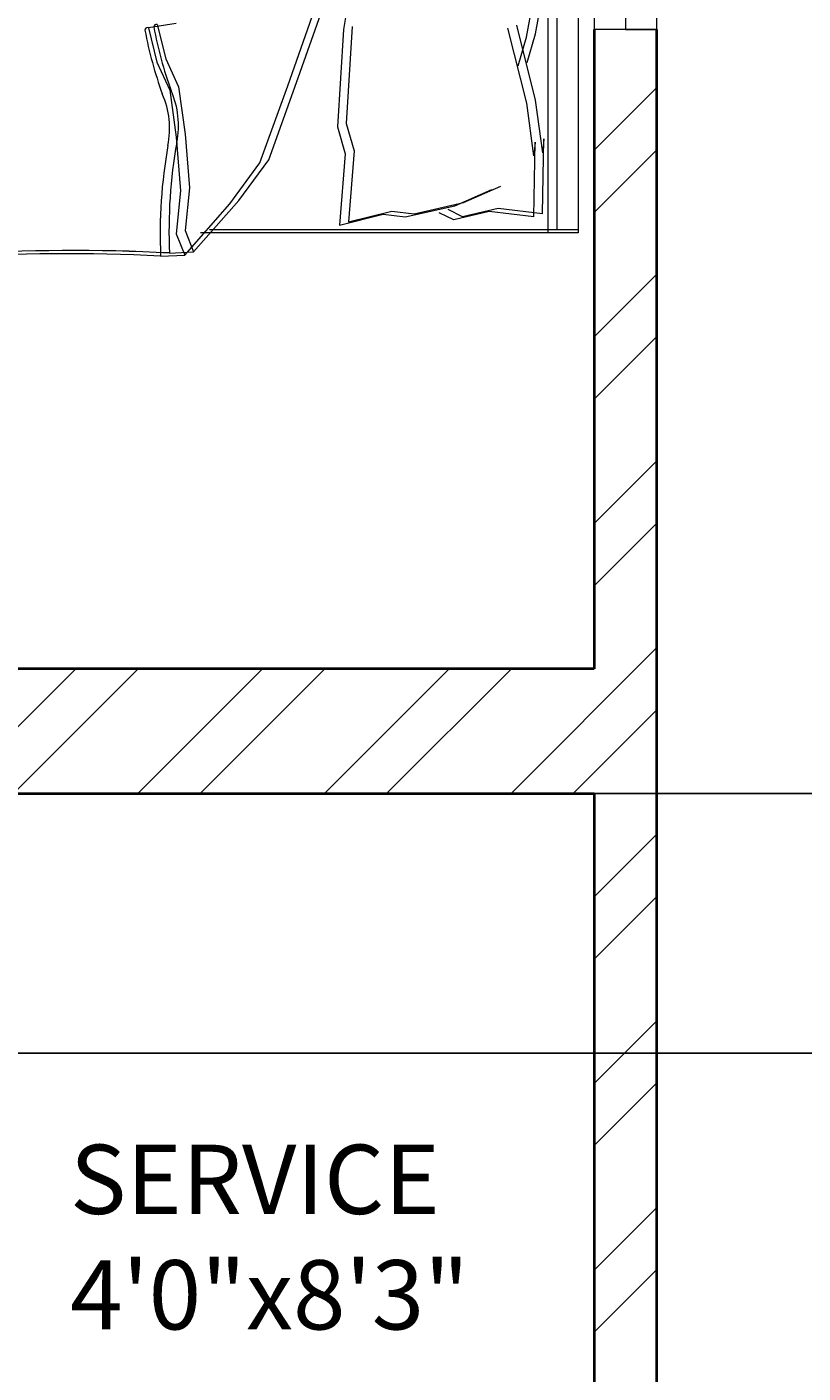
# Model space of a CAD drawing. Units: inches. Extents: x 1601 to 2297, y 1496 to 2631.
# Tile 31 of 57: x 2185 to 2241, y 2043 to 2141. Entities that reach past the tile are written whole.
import ezdxf

# ---------------------------------------------------------------- set-up
doc = ezdxf.new("R2010")
doc.units = ezdxf.units.IN
for name, color, linetype, lineweight in [('A-ANNO-DIMS', 2, 'Continuous', 18), ('A-AREA-IDEN', 7, 'Continuous', 18), ('A-FURN', 8, 'Continuous', 18), ('A-GLAZ', 161, 'Continuous', 20), ('A-WALL', 7, 'Continuous', 40), ('A-WALL-PATT', 215, 'Continuous', 13)]:
    doc.layers.add(name, color=color, linetype=linetype, lineweight=lineweight)
doc.styles.get("Standard").update_dxf_attribs({"font": 'arial.ttf'})
doc.dimstyles.get("Standard").update_dxf_attribs({"dimtxt": 0.18, "dimasz": 0.18, "dimexe": 0.18, "dimexo": 0.0625, "dimgap": 0.09, "dimtad": 0, "dimtih": 1, "dimtoh": 1, "dimdec": 4, "dimzin": 0, "dimdsep": 46, "dimtxsty": 'Standard', "dimcen": 0.09, "dimadec": 0, "dimazin": 0, "dimtfac": 1, "dimtdec": 4, "dimtofl": 0, "dimtmove": 0, "dimatfit": 3, "dimfxl": 1, "dimtolj": 1, "dimtzin": 0, "dimarcsym": 0})

# ---------------------------------------------------------------- blocks, each defined once
blk = doc.blocks.new('BED-DOUBLE')
for p, q in [((27.746, 52.867), (24.495, 49.162)), ((27.746, 52.867), (24.495, 49.162)), ((27.746, 52.867), (24.495, 49.162)), ((27.746, 52.867), (24.495, 49.162)), ((28.385, 53.096), (25.135, 49.39)), ((28.385, 53.096), (25.135, 49.39)), ((28.385, 53.096), (25.135, 49.39)), ((28.385, 53.096), (25.135, 49.39)), ((29.49, 52.947), (27.746, 52.867, 3.871)), ((29.49, 52.947), (27.746, 52.867, 3.871)), ((29.49, 52.947), (27.746, 52.867, 3.871)), ((29.49, 52.947), (27.746, 52.867, 3.871)), ((28.365, 51.33), (27.746, 52.867)), ((28.365, 51.33), (27.746, 52.867)), ((28.365, 51.33), (27.746, 52.867)), ((28.365, 51.33), (27.746, 52.867)), ((30.13, 53.175), (28.385, 53.096, 3.871)), ((30.13, 53.175), (28.385, 53.096, 3.871)), ((30.13, 53.175), (28.385, 53.096, 3.871)), ((30.13, 53.175), (28.385, 53.096, 3.871)), ((29.004, 51.559), (28.385, 53.096)), ((29.004, 51.558), (28.385, 53.096)), ((29.004, 51.559), (28.385, 53.096)), ((29.004, 51.558), (28.385, 53.096)), ((28.695, 48.461), (29.004, 51.559)), ((28.695, 48.461), (29.004, 51.559)), ((28.695, 48.461), (29.004, 51.558)), ((28.695, 48.461), (29.004, 51.558)), ((0, 51.494), (0.639, 51.493)), ((0, 3.475), (0, 51.494)), ((0, 51.494), (0.639, 51.493)), ((0, 3.475), (0, 51.494)), ((0, 51.265), (26.61, 51.265)), ((0, 51.265), (26.61, 51.265)), ((0, 51.265), (26.61, 51.265)), ((0, 51.265), (26.61, 51.265)), ((0.639, 51.494), (27.249, 51.494)), ((0.639, 51.494), (27.249, 51.494)), ((0.639, 51.493), (27.249, 51.493)), ((0.639, 51.493), (27.249, 51.493)), ((1.533, 3.475), (1.533, 51.265)), ((1.533, 3.475), (1.533, 51.265)), ((1.533, 3.475), (1.533, 51.265)), ((1.533, 3.475), (1.533, 51.265)), ((2.173, 3.703), (2.173, 51.494)), ((2.173, 3.703), (2.173, 51.494)), ((2.173, 3.703), (2.173, 51.493)), ((2.173, 3.703), (2.173, 51.493)), ((6.407, 49.961), (8.977, 50.557)), ((6.407, 49.961), (8.977, 50.557)), ((6.407, 49.961), (8.977, 50.556)), ((6.407, 49.961), (8.977, 50.556)), ((8.977, 50.557), (10.024, 50.043)), ((8.977, 50.557), (10.024, 50.043)), ((8.977, 50.556), (10.024, 50.042)), ((8.977, 50.556), (10.024, 50.042)), ((16.573, 50.698), (13.434, 49.923)), ((16.573, 50.698), (13.434, 49.922)), ((16.573, 50.698), (13.434, 49.923)), ((16.573, 50.698), (13.434, 49.922)), ((17.212, 50.926), (14.073, 50.151)), ((17.212, 50.926), (14.073, 50.151)), ((17.212, 50.926), (14.073, 50.151)), ((17.212, 50.926), (14.073, 50.151)), ((16.169, 45.566), (16.573, 50.698)), ((16.169, 45.566), (16.573, 50.698)), ((16.169, 45.566), (16.573, 50.698)), ((16.169, 45.566), (16.573, 50.698)), ((16.808, 45.795), (17.212, 50.926)), ((16.808, 45.794), (17.212, 50.926)), ((16.808, 45.795), (17.212, 50.926)), ((16.808, 45.794), (17.212, 50.926)), ((28.055, 48.233), (28.365, 51.33)), ((28.055, 48.233), (28.365, 51.33)), ((28.055, 48.233), (28.365, 51.33)), ((28.055, 48.233), (28.365, 51.33)), ((2.557, 50.112), (2.46, 44.709)), ((2.557, 50.112), (2.46, 44.709)), ((2.557, 50.111), (2.46, 44.709)), ((2.557, 50.111), (2.46, 44.709)), ((2.557, 50.112), (5.768, 49.733)), ((2.557, 50.112), (5.768, 49.733)), ((2.557, 50.111), (5.768, 49.733)), ((2.557, 50.111), (5.768, 49.733)), ((3.196, 50.34), (3.099, 44.938)), ((3.196, 50.34), (3.099, 44.938)), ((3.196, 50.34), (3.099, 44.938)), ((3.196, 50.34), (3.099, 44.938)), ((3.196, 50.34), (6.407, 49.961)), ((3.196, 50.34), (6.407, 49.961)), ((3.196, 50.34), (6.407, 49.961)), ((3.196, 50.34), (6.407, 49.961)), ((5.768, 49.733), (8.338, 50.328)), ((5.768, 49.733), (8.338, 50.328)), ((5.768, 49.733), (8.338, 50.328)), ((5.768, 49.733), (8.338, 50.328)), ((11.829, 50.112), (8.257, 49.309)), ((11.829, 50.112), (8.257, 49.309)), ((11.829, 50.112), (8.257, 49.309)), ((11.829, 50.112), (8.257, 49.309)), ((8.338, 50.328), (9.384, 49.814)), ((8.338, 50.328), (9.384, 49.814)), ((8.338, 50.328), (9.384, 49.814)), ((8.338, 50.328), (9.384, 49.814)), ((12.468, 50.34), (8.896, 49.538)), ((12.468, 50.34), (8.896, 49.537)), ((12.468, 50.34), (8.896, 49.538)), ((12.468, 50.34), (8.896, 49.537)), ((13.434, 49.923), (11.829, 50.112)), ((13.434, 49.922), (11.829, 50.112)), ((13.434, 49.923), (11.829, 50.112)), ((13.434, 49.922), (11.829, 50.112)), ((14.073, 50.151), (12.468, 50.34)), ((14.073, 50.151), (12.468, 50.34)), ((14.073, 50.151), (12.468, 50.34)), ((14.073, 50.151), (12.468, 50.34)), ((8.257, 49.309), (5.578, 48.128)), ((8.257, 49.309), (5.578, 48.128)), ((8.257, 49.309), (5.578, 48.128)), ((8.257, 49.309), (5.578, 48.128)), ((8.896, 49.538), (6.218, 48.356)), ((8.896, 49.538), (6.218, 48.356)), ((8.896, 49.537), (6.218, 48.356)), ((8.896, 49.537), (6.218, 48.356)), ((24.495, 49.162), (22.329, 46.219)), ((24.495, 49.162), (22.329, 46.219)), ((24.495, 49.162), (22.329, 46.219)), ((24.495, 49.162), (22.329, 46.219)), ((25.135, 49.39), (22.968, 46.448)), ((25.135, 49.39), (22.968, 46.448)), ((25.135, 49.39), (22.968, 46.448)), ((25.135, 49.39), (22.968, 46.448)), ((28.365, 44.361), (28.055, 48.233)), ((28.365, 44.361), (28.055, 48.233)), ((28.365, 44.361), (28.055, 48.233)), ((28.365, 44.361), (28.055, 48.233)), ((29.004, 44.589), (28.695, 48.461)), ((29.004, 44.589), (28.695, 48.461)), ((29.004, 44.589), (28.695, 48.461)), ((29.004, 44.589), (28.695, 48.461)), ((2.46, 44.709), (2.542, 45.712)), ((2.46, 44.709), (2.542, 45.712)), ((2.46, 44.709), (2.542, 45.712)), ((2.46, 44.709), (2.542, 45.712)), ((2.542, 45.712), (3.069, 41.914)), ((2.542, 45.712), (3.069, 41.914)), ((2.542, 45.712), (3.069, 41.914)), ((2.542, 45.712), (3.069, 41.914)), ((3.099, 44.938), (3.181, 45.941)), ((3.099, 44.938), (3.181, 45.941)), ((3.099, 44.938), (3.181, 45.94)), ((3.099, 44.938), (3.181, 45.94)), ((3.181, 45.941), (3.709, 42.143)), ((3.181, 45.941), (3.709, 42.143)), ((3.181, 45.94), (3.709, 42.142)), ((3.181, 45.94), (3.709, 42.142)), ((17.365, 43.834), (16.808, 45.795)), ((17.365, 43.834), (16.808, 45.795)), ((17.365, 43.834), (16.808, 45.794)), ((17.365, 43.834), (16.808, 45.794)), ((22.329, 46.219), (20.316, 40.644)), ((22.329, 46.219), (20.316, 40.644)), ((22.329, 46.219), (20.317, 40.644)), ((22.329, 46.219), (20.317, 40.644)), ((22.968, 46.448), (20.956, 40.872)), ((22.968, 46.448), (20.956, 40.872)), ((22.968, 46.448), (20.956, 40.872)), ((22.968, 46.448), (20.956, 40.872)), ((16.726, 43.606), (16.169, 45.566)), ((16.726, 43.606), (16.169, 45.566)), ((16.726, 43.606), (16.169, 45.566)), ((16.726, 43.606), (16.169, 45.566)), ((16.934, 36.824), (17.365, 43.834)), ((16.934, 36.824), (17.365, 43.834)), ((16.934, 36.824), (17.365, 43.834)), ((16.934, 36.824), (17.365, 43.834)), ((28.829, 40.954), (28.365, 44.361)), ((28.829, 40.953), (28.365, 44.361)), ((28.829, 40.954), (28.365, 44.361)), ((28.829, 40.953), (28.365, 44.361)), ((29.468, 41.182), (29.004, 44.589)), ((29.469, 41.182), (29.004, 44.589)), ((29.468, 41.182), (29.004, 44.589)), ((29.469, 41.182), (29.004, 44.589)), ((16.295, 36.596), (16.726, 43.606)), ((16.295, 36.596), (16.726, 43.606)), ((16.295, 36.596), (16.726, 43.606)), ((16.295, 36.596), (16.726, 43.606)), ((3.069, 41.914), (4.422, 36.495)), ((3.069, 41.914), (4.422, 36.495)), ((3.069, 41.914), (4.422, 36.495)), ((3.069, 41.914), (4.422, 36.495)), ((3.709, 42.143), (5.061, 36.723)), ((3.709, 42.143), (5.061, 36.723)), ((3.709, 42.142), (5.061, 36.723)), ((3.709, 42.142), (5.061, 36.723)), ((20.956, 40.872), (18.022, 32.534)), ((20.956, 40.872), (18.022, 32.534)), ((20.956, 40.872), (18.022, 32.534)), ((20.956, 40.872), (18.022, 32.534)), ((29.758, 38.94), (28.829, 40.954)), ((29.758, 38.94), (28.829, 40.954)), ((29.758, 38.94), (28.829, 40.953)), ((29.758, 38.94), (28.829, 40.953)), ((30.397, 39.169), (29.468, 41.182)), ((30.397, 39.169), (29.468, 41.182)), ((30.397, 39.168), (29.469, 41.182)), ((30.397, 39.168), (29.469, 41.182)), ((20.316, 40.644), (17.383, 32.306)), ((20.317, 40.644), (17.383, 32.306)), ((20.316, 40.644), (17.383, 32.306)), ((20.317, 40.644), (17.383, 32.306)), ((3.673, 39.2), (3.078, 37.135)), ((3.673, 39.2), (3.078, 37.135)), ((3.673, 39.2), (3.078, 37.135)), ((3.673, 39.2), (3.078, 37.135)), ((4.313, 39.428), (3.717, 37.363)), ((4.313, 39.428), (3.717, 37.363)), ((4.313, 39.428), (3.718, 37.363)), ((4.313, 39.428), (3.718, 37.363)), ((30.377, 36.462), (29.758, 38.94)), ((30.377, 36.462), (29.758, 38.94)), ((30.377, 36.462), (29.758, 38.94)), ((30.377, 36.462), (29.758, 38.94)), ((31.016, 36.691), (30.397, 39.169)), ((31.016, 36.691), (30.397, 39.169)), ((31.016, 36.691), (30.397, 39.168)), ((31.016, 36.691), (30.397, 39.168)), ((3.078, 37.135), (2.537, 34.204)), ((3.078, 37.135), (2.537, 34.204)), ((3.078, 37.135), (2.537, 34.204)), ((3.078, 37.135), (2.537, 34.204)), ((3.717, 37.363), (3.176, 34.433)), ((3.718, 37.363), (3.176, 34.433)), ((3.717, 37.363), (3.176, 34.433)), ((3.718, 37.363), (3.176, 34.433)), ((16.268, 32.792), (16.934, 36.824)), ((16.268, 32.792), (16.934, 36.824)), ((16.268, 32.792), (16.934, 36.824)), ((16.268, 32.792), (16.934, 36.824)), ((29.004, 36.381), (31.016, 36.691)), ((29.004, 36.381), (31.016, 36.691)), ((29.004, 36.381), (31.016, 36.691)), ((29.004, 36.381), (31.016, 36.691))]:
    blk.add_line(p, q)
for centre, radius, start, end in [((-6.656, 51.327), 36.183, 349.87628, 2.56571), ((-6.656, 51.327), 36.183, 349.87628, 2.56571), ((-6.656, 51.327), 36.183, 349.87628, 2.56571), ((-6.656, 51.327), 36.183, 349.87628, 2.56571), ((36.315, 182.266), 129.499, 266.97912, 273.83645), ((36.315, 182.265), 129.499, 266.97912, 273.83645), ((36.315, 182.266), 129.499, 266.97912, 273.83645), ((36.315, 182.265), 129.499, 266.97912, 273.83645), ((-6.017, 51.555), 36.183, 349.87628, 2.56571), ((-6.017, 51.555), 36.183, 349.87628, 2.56571), ((-6.017, 51.555), 36.183, 349.87628, 2.56571), ((-6.017, 51.555), 36.183, 349.87628, 2.56571), ((36.954, 182.494), 129.499, 266.97912, 273.83645), ((36.954, 182.494), 129.499, 266.97912, 273.83645), ((36.954, 182.494), 129.499, 266.97912, 273.83645), ((36.954, 182.494), 129.499, 266.97912, 273.83645), ((35.066, 43.743), 6.224, 168.6608, 203.73842), ((35.066, 43.743), 6.224, 168.6608, 203.73842), ((35.066, 43.743), 6.224, 168.6608, 203.73842), ((35.066, 43.743), 6.224, 168.6608, 203.73842), ((35.705, 43.972), 6.224, 168.6608, 203.73842), ((35.705, 43.971), 6.224, 168.6608, 203.73842), ((35.705, 43.972), 6.224, 168.6608, 203.73842), ((35.705, 43.971), 6.224, 168.6608, 203.73842), ((1.482, 31.154), 29.654, 10.66171, 19.88058), ((1.482, 31.154), 29.654, 10.66171, 19.88058), ((1.482, 31.153), 29.654, 10.66171, 19.88058), ((1.482, 31.153), 29.654, 10.66171, 19.88058), ((2.121, 31.382), 29.654, 10.66171, 19.88058), ((2.121, 31.382), 29.654, 10.66171, 19.88058), ((2.121, 31.382), 29.654, 10.66171, 19.88058), ((2.121, 31.382), 29.654, 10.66171, 19.88058), ((30.439, 36.636), 0.185, 250.24637, 1.13765), ((30.439, 36.636), 0.185, 250.24637, 1.13765), ((30.439, 36.636), 0.185, 250.24637, 1.13765), ((30.439, 36.636), 0.185, 250.24637, 1.13765), ((31.079, 36.864), 0.185, 250.24637, 1.13765), ((31.079, 36.864), 0.185, 250.24637, 1.13765), ((31.079, 36.864), 0.185, 250.24637, 1.13765), ((31.079, 36.864), 0.185, 250.24637, 1.13765)]:
    blk.add_arc(centre, radius, start, end)
blk = doc.blocks.new('WIN-60IN-JAMB4P5')
for p, q in [((0, 60), (4.5, 60)), ((0, 60), (0, 0)), ((4.5, 60), (2.25, 60)), ((2.25, 60), (2.25, 0)), ((4.5, 60), (4.5, 0)), ((4.5, 0), (0, 0)), ((2.25, 0), (4.5, 0))]:
    blk.add_line(p, q)
blk = doc.blocks.new('*D29')
at = {"layer": 'A-ANNO-DIMS', "color": 0, "lineweight": -2, "transparency": 16777216}
for p, q in [((2230.6, 2532.325), (2279.267, 2532.325)), ((2279.087, 2532.145), (2279.087, 2084.007)), ((2279.087, 1635.505), (2279.087, 2083.643)), ((2230.6, 1635.325), (2279.267, 1635.325))]:
    blk.add_line(p, q, dxfattribs=at)
at = {"layer": 'A-ANNO-DIMS', "color": 0, "transparency": 16777216}
for points in [[(2279.057, 2532.145), (2279.117, 2532.145), (2279.087, 2532.325)], [(2279.057, 1635.505), (2279.117, 1635.505), (2279.087, 1635.325)]]:
    blk.add_solid(points, dxfattribs=at)
at = {"layer": 'Defpoints', "color": 0, "transparency": 16777216}
for p in [(2230.537, 2532.325), (2279.087, 2532.325), (2230.537, 1635.325)]:
    blk.add_point(p, dxfattribs=at)
at = {"layer": 'A-ANNO-DIMS', "color": 0, "transparency": 16777216, "insert": (2279.087, 2083.825), "char_height": 0.18, "attachment_point": 5}
blk.add_mtext('\\A1;897', dxfattribs=at)
blk = doc.blocks.new('*D37')
at = {"layer": 'A-ANNO-DIMS', "color": 0, "lineweight": -2, "transparency": 16777216}
for p, q in [((2040.1, 2085.325), (2279.267, 2085.325)), ((2279.087, 2085.145), (2279.087, 2076.132)), ((2279.087, 2066.755), (2279.087, 2075.768)), ((2040.1, 2066.575), (2279.267, 2066.575))]:
    blk.add_line(p, q, dxfattribs=at)
at = {"layer": 'A-ANNO-DIMS', "color": 0, "transparency": 16777216}
for points in [[(2279.057, 2085.145), (2279.117, 2085.145), (2279.087, 2085.325)], [(2279.057, 2066.755), (2279.117, 2066.755), (2279.087, 2066.575)]]:
    blk.add_solid(points, dxfattribs=at)
at = {"layer": 'Defpoints', "color": 0, "transparency": 16777216}
for p in [(2040.037, 2085.325), (2279.087, 2085.325), (2040.037, 2066.575)]:
    blk.add_point(p, dxfattribs=at)
at = {"layer": 'A-ANNO-DIMS', "color": 0, "transparency": 16777216, "insert": (2279.087, 2075.95), "char_height": 0.18, "attachment_point": 5}
blk.add_mtext('\\A1;18.75', dxfattribs=at)

msp = doc.modelspace()

# ---------------------------------------------------------------- hatches: boundary and pattern name
at = {"layer": 'A-WALL-PATT'}
h = msp.add_hatch(dxfattribs=at)
h.set_pattern_fill('ANSI32', color=256)
h.paths.add_polyline_path([(1842.0336, 2528.0767), (1842.0336, 2532.3254), (1686.0373, 2532.3254), (1686.0373, 2492.9493), (1695.0373, 2492.9493), (1695.0373, 2523.3254), (1827.0373, 2523.3254), (1827.0373, 2416.8254), (1834.6225, 2416.8254), (1834.6225, 2419.0754), (1834.6225, 2421.3254), (1831.5373, 2421.3254), (1831.5373, 2523.3254), (1842.0336, 2523.3254)])
h.paths.add_polyline_path([(1695.0373, 2432.9493), (1686.0373, 2432.9493), (1686.0373, 2325.989), (1695.0373, 2325.989), (1695.0373, 2347.8254), (1827.0373, 2347.8254), (1827.0373, 2287.8254), (1823.2991, 2287.8254), (1823.2991, 2283.3254), (1847.9422, 2283.3254), (1847.9422, 2285.5754), (1847.9422, 2287.8254), (1831.5373, 2287.8254), (1831.5373, 2347.8254), (1846.9946, 2347.8254), (1846.9946, 2350.0754), (1846.9946, 2352.3254), (1695.0373, 2352.3254)])
h.paths.add_polyline_path([(1807.1169, 1573.5395), (2055.0405, 1573.5395), (2055.0405, 1610.6322), (1807.1169, 1610.6322)], flags=9)
h.paths.add_polyline_path([(1841.1631, 1712.7967), (1870.3957, 1712.7967), (1870.3957, 1731.454), (1841.1631, 1731.454)], flags=9)
h.paths.add_polyline_path([(2144.3862, 1772.185), (2191.0233, 1772.185), (2191.0233, 1790.8423), (2144.3862, 1790.8423)], flags=9)
h.paths.add_polyline_path([(2143.0128, 1827.3312), (2177.9958, 1827.3312), (2177.9958, 1845.9886), (2143.0128, 1845.9886)], flags=9)
h.paths.add_polyline_path([(2041.2439, 1833.5691), (2070.8516, 1833.5691), (2070.8516, 1852.2264), (2041.2439, 1852.2264)], flags=9)
h.paths.add_polyline_path([(2097.2791, 1947.0598), (2134.2061, 1947.0598), (2134.2061, 1965.7171), (2097.2791, 1965.7171)], flags=9)
h.paths.add_polyline_path([(2214.995, 1904.3124), (2214.995, 1942.2899), (2196.3376, 1942.2899), (2196.3376, 1904.3124)], flags=9)
h.paths.add_polyline_path([(2186.6284, 2043.8031), (2219.7935, 2043.8031), (2219.7935, 2062.4605), (2186.6284, 2062.4605)], flags=9)
h.paths.add_polyline_path([(2064.0877, 2031.616), (2097.4949, 2031.616), (2097.4949, 2050.2734), (2064.0877, 2050.2734)], flags=9)
h.paths.add_polyline_path([(1973.1349, 1986.0688), (2008.4009, 1986.0688), (2008.4009, 2004.7261), (1973.1349, 2004.7261)], flags=9)
h.paths.add_polyline_path([(1976.3676, 2106.9635), (2005.7469, 2106.9635), (2005.7469, 2125.6209), (1976.3676, 2125.6209)], flags=9)
h.paths.add_polyline_path([(1991.7852, 2180.4863), (2027.0513, 2180.4863), (2027.0513, 2199.1437), (1991.7852, 2199.1437)], flags=9)
h.paths.add_polyline_path([(2106.1801, 2187.9359), (2152.2101, 2187.9359), (2152.2101, 2206.5932), (2106.1801, 2206.5932)], flags=9)
h.paths.add_polyline_path([(2148.6686, 2262.2542), (2182.318, 2262.2542), (2182.318, 2280.9115), (2148.6686, 2280.9115)], flags=9)
h.paths.add_polyline_path([(2041.6327, 2252.8147), (2071.2405, 2252.8147), (2071.2405, 2271.4721), (2041.6327, 2271.4721)], flags=9)
h.paths.add_polyline_path([(2063.9734, 2375.4265), (2100.9004, 2375.4265), (2100.9004, 2394.0839), (2063.9734, 2394.0839)], flags=9)
h.paths.add_polyline_path([(2216.4955, 2330.9748), (2216.4955, 2370.2654), (2197.8381, 2370.2654), (2197.8381, 2330.9748)], flags=9)
h.paths.add_polyline_path([(2179.1416, 2485.8687), (2212.3067, 2485.8687), (2212.3067, 2504.5261), (2179.1416, 2504.5261)], flags=9)
h.paths.add_polyline_path([(2078.7442, 2471.1516), (2112.1514, 2471.1516), (2112.1514, 2489.809), (2078.7442, 2489.809)], flags=9)
h.paths.add_polyline_path([(1915.9631, 2329.4668), (1952.8902, 2329.4668), (1952.8902, 2348.1241), (1915.9631, 2348.1241)], flags=9)
h.paths.add_polyline_path([(1904.3189, 2499.6709), (1940.4512, 2499.6709), (1940.4512, 2518.3282), (1904.3189, 2518.3282)], flags=9)
h.paths.add_polyline_path([(1892.3665, 2100.4595), (1925.6374, 2100.4595), (1925.6374, 2119.1169), (1892.3665, 2119.1169)], flags=9)
h.paths.add_polyline_path([(1909.2984, 1805.9631), (1946.2254, 1805.9631), (1946.2254, 1824.6205), (1909.2984, 1824.6205)], flags=9)
h.paths.add_polyline_path([(1934.6056, 1658.616), (1970.738, 1658.616), (1970.738, 1677.2733), (1934.6056, 1677.2733)], flags=9)
h.paths.add_polyline_path([(1711.2052, 1789.8902), (1750.0456, 1789.8902), (1750.0456, 1808.5476), (1711.2052, 1808.5476)], flags=9)
h.paths.add_polyline_path([(1742.7874, 1854.6743), (1771.9449, 1854.6743), (1771.9449, 1873.3317), (1742.7874, 1873.3317)], flags=9)
h.paths.add_polyline_path([(1807.3592, 1997.7912), (1850.1116, 1997.7912), (1850.1116, 2016.4486), (1807.3592, 2016.4486)], flags=9)
h.paths.add_polyline_path([(1717.4579, 2237.7844), (1760.2103, 2237.7844), (1760.2103, 2256.4417), (1717.4579, 2256.4417)], flags=9)
h.paths.add_polyline_path([(1780.9285, 2324.0623), (1810.086, 2324.0623), (1810.086, 2342.7197), (1780.9285, 2342.7197)], flags=25)
h.paths.add_polyline_path([(1837.696, 2449.2024), (1866.9286, 2449.2024), (1866.9286, 2467.8598), (1837.696, 2467.8598)], flags=9)
h.paths.add_polyline_path([(1712.7752, 2484.9404), (1751.6156, 2484.9404), (1751.6156, 2503.5977), (1712.7752, 2503.5977)], flags=25)
h = msp.add_hatch(dxfattribs=at)
h.set_pattern_fill('ANSI32', color=256)
h.paths.add_polyline_path([(1973.9371, 2211.3254), (1893.0373, 2211.3254), (1893.0373, 2287.8254), (1884.6167, 2287.8254), (1884.6167, 2285.5754), (1884.6167, 2283.3254), (1888.5373, 2283.3254), (1888.5373, 2145.3254), (1695.0373, 2145.3254), (1695.0373, 2173.8724), (1690.5373, 2173.8724), (1686.0373, 2173.8724), (1686.0373, 2136.3254), (1722.5687, 2136.3254), (1722.5687, 2117.4352), (1731.5687, 2117.4352), (1731.5687, 2136.3254), (1893.0373, 2136.3254), (1893.0373, 2202.3254), (1959.0373, 2202.3254), (1959.0373, 2182.1303), (1968.0373, 2182.1303), (1968.0373, 2202.3254), (1973.9371, 2202.3254)])
h.paths.add_polyline_path([(2094.0373, 2274.6364), (2096.4294, 2274.6364), (2096.4294, 2276.8864), (2096.4294, 2279.1364), (2094.0373, 2279.1364), (2094.0373, 2290.8254), (2094.0373, 2295.3254), (2089.5373, 2295.3254), (2089.5373, 2230.8254), (2035.5373, 2230.8254), (2035.5373, 2299.8254), (2031.0373, 2299.8254), (2031.0373, 2211.3254), (2023.0065, 2211.3254), (2023.0065, 2202.3254), (2031.0373, 2202.3254), (2031.0373, 2140.8254), (1968.0373, 2140.8254), (1968.0373, 2145.9106), (1963.5373, 2145.9106), (1959.0373, 2145.9106), (1959.0373, 2116.839), (1963.5373, 2116.839), (1968.0373, 2116.839), (1968.0373, 2131.8254), (2031.0373, 2131.8254), (2031.0373, 2094.3254), (2031.0373, 2085.3254), (2031.0373, 2056.8254), (1968.0373, 2056.8254), (1968.0373, 2070.4947), (1963.5373, 2070.4947), (1959.0373, 2070.4947), (1959.0373, 2040.3029), (1968.0373, 2040.3029), (1968.0373, 2047.8254), (2031.0373, 2047.8254), (2031.0373, 1983.3254), (2031.0373, 1978.8254), (2021.1979, 1978.8254), (2021.1979, 1974.3254), (2031.0373, 1974.3254), (2031.0373, 1954.3528), (2035.5373, 1954.3528), (2035.5373, 1974.3254), (2035.5373, 1981.8254), (2055.5513, 1981.8254), (2055.5513, 1986.3254), (2035.5373, 1986.3254), (2035.5373, 2047.8254), (2040.0373, 2047.8254), (2040.0373, 2085.3254), (2040.0373, 2094.3254), (2040.0373, 2140.8254), (2035.5373, 2140.8254), (2035.5373, 2226.3254), (2089.5373, 2226.3254), (2094.0373, 2226.3254)])
h.paths.add_polyline_path([(2226.0373, 2230.8254), (2134.5373, 2230.8254), (2134.5373, 2233.5437), (2130.0373, 2233.5437), (2130.0373, 2226.3254), (2134.5373, 2226.3254), (2226.0373, 2226.3254)])
h.paths.add_polyline_path([(1807.1169, 1573.5395), (2055.0405, 1573.5395), (2055.0405, 1610.6322), (1807.1169, 1610.6322)], flags=9)
h.paths.add_polyline_path([(1841.1631, 1712.7967), (1870.3957, 1712.7967), (1870.3957, 1731.454), (1841.1631, 1731.454)], flags=9)
h.paths.add_polyline_path([(2144.3862, 1772.185), (2191.0233, 1772.185), (2191.0233, 1790.8423), (2144.3862, 1790.8423)], flags=9)
h.paths.add_polyline_path([(2143.0128, 1827.3312), (2177.9958, 1827.3312), (2177.9958, 1845.9886), (2143.0128, 1845.9886)], flags=9)
h.paths.add_polyline_path([(2041.2439, 1833.5691), (2070.8516, 1833.5691), (2070.8516, 1852.2264), (2041.2439, 1852.2264)], flags=9)
h.paths.add_polyline_path([(2097.2791, 1947.0598), (2134.2061, 1947.0598), (2134.2061, 1965.7171), (2097.2791, 1965.7171)], flags=9)
h.paths.add_polyline_path([(2214.995, 1904.3124), (2214.995, 1942.2899), (2196.3376, 1942.2899), (2196.3376, 1904.3124)], flags=9)
h.paths.add_polyline_path([(2186.6284, 2043.8031), (2219.7935, 2043.8031), (2219.7935, 2062.4605), (2186.6284, 2062.4605)], flags=9)
h.paths.add_polyline_path([(2064.0877, 2031.616), (2097.4949, 2031.616), (2097.4949, 2050.2734), (2064.0877, 2050.2734)], flags=9)
h.paths.add_polyline_path([(1973.1349, 1986.0688), (2008.4009, 1986.0688), (2008.4009, 2004.7261), (1973.1349, 2004.7261)], flags=25)
h.paths.add_polyline_path([(1976.3676, 2106.9635), (2005.7469, 2106.9635), (2005.7469, 2125.6209), (1976.3676, 2125.6209)], flags=25)
h.paths.add_polyline_path([(1991.7852, 2180.4863), (2027.0513, 2180.4863), (2027.0513, 2199.1437), (1991.7852, 2199.1437)], flags=25)
h.paths.add_polyline_path([(2106.1801, 2187.9359), (2152.2101, 2187.9359), (2152.2101, 2206.5932), (2106.1801, 2206.5932)], flags=9)
h.paths.add_polyline_path([(2148.6686, 2262.2542), (2182.318, 2262.2542), (2182.318, 2280.9115), (2148.6686, 2280.9115)], flags=9)
h.paths.add_polyline_path([(2041.6327, 2252.8147), (2071.2405, 2252.8147), (2071.2405, 2271.4721), (2041.6327, 2271.4721)], flags=25)
h.paths.add_polyline_path([(2063.9734, 2375.4265), (2100.9004, 2375.4265), (2100.9004, 2394.0839), (2063.9734, 2394.0839)], flags=9)
h.paths.add_polyline_path([(2216.4955, 2330.9748), (2216.4955, 2370.2654), (2197.8381, 2370.2654), (2197.8381, 2330.9748)], flags=9)
h.paths.add_polyline_path([(2179.1416, 2485.8687), (2212.3067, 2485.8687), (2212.3067, 2504.5261), (2179.1416, 2504.5261)], flags=9)
h.paths.add_polyline_path([(2078.7442, 2471.1516), (2112.1514, 2471.1516), (2112.1514, 2489.809), (2078.7442, 2489.809)], flags=9)
h.paths.add_polyline_path([(1915.9631, 2329.4668), (1952.8902, 2329.4668), (1952.8902, 2348.1241), (1915.9631, 2348.1241)], flags=9)
h.paths.add_polyline_path([(1904.3189, 2499.6709), (1940.4512, 2499.6709), (1940.4512, 2518.3282), (1904.3189, 2518.3282)], flags=9)
h.paths.add_polyline_path([(1892.3665, 2100.4595), (1925.6374, 2100.4595), (1925.6374, 2119.1169), (1892.3665, 2119.1169)], flags=9)
h.paths.add_polyline_path([(1909.2984, 1805.9631), (1946.2254, 1805.9631), (1946.2254, 1824.6205), (1909.2984, 1824.6205)], flags=9)
h.paths.add_polyline_path([(1934.6056, 1658.616), (1970.738, 1658.616), (1970.738, 1677.2733), (1934.6056, 1677.2733)], flags=9)
h.paths.add_polyline_path([(1711.2052, 1789.8902), (1750.0456, 1789.8902), (1750.0456, 1808.5476), (1711.2052, 1808.5476)], flags=9)
h.paths.add_polyline_path([(1742.7874, 1854.6743), (1771.9449, 1854.6743), (1771.9449, 1873.3317), (1742.7874, 1873.3317)], flags=9)
h.paths.add_polyline_path([(1807.3592, 1997.7912), (1850.1116, 1997.7912), (1850.1116, 2016.4486), (1807.3592, 2016.4486)], flags=9)
h.paths.add_polyline_path([(1717.4579, 2237.7844), (1760.2103, 2237.7844), (1760.2103, 2256.4417), (1717.4579, 2256.4417)], flags=25)
h.paths.add_polyline_path([(1780.9285, 2324.0623), (1810.086, 2324.0623), (1810.086, 2342.7197), (1780.9285, 2342.7197)], flags=9)
h.paths.add_polyline_path([(1837.696, 2449.2024), (1866.9286, 2449.2024), (1866.9286, 2467.8598), (1837.696, 2467.8598)], flags=9)
h.paths.add_polyline_path([(1712.7752, 2484.9404), (1751.6156, 2484.9404), (1751.6156, 2503.5977), (1712.7752, 2503.5977)], flags=9)
h = msp.add_hatch(dxfattribs=at)
h.set_pattern_fill('ANSI32', color=256)
h.paths.add_polyline_path([(2230.5373, 1861.8254), (2182.5373, 1861.8254), (2182.5373, 1885.3637), (2178.0373, 1885.3637), (2178.0373, 1861.8254), (2166.0373, 1861.8254), (2134.5373, 1861.8254), (2130.0373, 1861.8254), (2130.0373, 1841.4682), (2126.8833, 1841.4682), (2126.8833, 1836.9682), (2130.0373, 1836.9682), (2130.0373, 1822.7302), (2134.5373, 1822.7302), (2134.5373, 1857.3254), (2166.0373, 1857.3254), (2226.0373, 1857.3254), (2226.0373, 1846.1155), (2230.5373, 1846.1155)])
h.paths.add_polyline_path([(2226.0373, 1797.3254), (2134.5373, 1797.3254), (2134.5373, 1800.6636), (2132.2873, 1800.6636), (2130.0373, 1800.6636), (2130.0373, 1797.3254), (2130.0373, 1792.8254), (2167.7264, 1792.8254), (2226.0373, 1792.8254)])
h.paths.add_polyline_path([(2230.5373, 1822.1155), (2226.0373, 1822.1155), (2226.0373, 1760.8563), (2230.5373, 1760.8563)])
h.paths.add_polyline_path([(2230.5373, 1700.8563), (2226.0373, 1700.8563), (2226.0373, 1644.3254), (2140.2517, 1644.3254), (2140.2517, 1635.3254), (2230.5373, 1635.3254)])
h.paths.add_polyline_path([(2080.2517, 1639.8254), (2080.2517, 1644.3254), (2035.5373, 1644.3254), (2035.5373, 1792.8254), (2094.0373, 1792.8254), (2094.0373, 1797.3254), (2094.0373, 1836.9682), (2097.1057, 1836.9682), (2097.1057, 1839.2182), (2097.1057, 1841.4682), (2094.0373, 1841.4682), (2094.0373, 1862.2276), (2089.5373, 1862.2276), (2089.5373, 1797.3254), (2035.5373, 1797.3254), (2035.5373, 1857.3254), (2035.5373, 1885.0916), (2031.0373, 1885.0916), (2031.0373, 1710.3254), (2012.329, 1710.3254), (2012.329, 1701.3254), (2031.0373, 1701.3254), (2031.0373, 1644.3254), (2031.0373, 1635.3254), (2080.2517, 1635.3254)])
h.paths.add_polyline_path([(1836.0373, 1653.2033), (1842.6171, 1653.2033), (1842.6171, 1657.7033), (1842.6171, 1662.2033), (1831.5373, 1662.2033), (1831.5373, 1764.2033), (1835.3881, 1764.2033), (1835.3881, 1766.4533), (1835.3881, 1768.7033), (1831.5373, 1768.7033), (1827.0373, 1768.7033), (1827.0373, 1662.2033), (1827.0373, 1635.3254), (1836.0373, 1635.3254)])
h.paths.add_polyline_path([(1893.0373, 1701.3254), (1907.193, 1701.3254), (1907.193, 1705.8254), (1907.193, 1710.3254), (1893.0373, 1710.3254), (1893.0373, 1819.8254), (1882.6444, 1819.8254), (1882.6444, 1817.5754), (1882.6444, 1815.3254), (1888.5373, 1815.3254), (1888.5373, 1662.2033), (1884.0373, 1662.2033), (1866.6171, 1662.2033), (1866.6171, 1653.2033), (1882.391, 1653.2033), (1884.0373, 1653.2033), (1884.0373, 1635.3254), (1893.0373, 1635.3254)])
h.paths.add_polyline_path([(1739.3335, 1639.8254), (1739.3335, 1644.3254), (1695.0373, 1644.3254), (1695.0373, 1702.0135), (1690.5373, 1702.0135), (1686.0373, 1702.0135), (1686.0373, 1635.3254), (1739.3335, 1635.3254)])
h.paths.add_polyline_path([(1827.0373, 1644.3254), (1799.3335, 1644.3254), (1799.3335, 1635.3254), (1827.0373, 1635.3254)])
h.paths.add_polyline_path([(1695.0373, 1815.3254), (1849.2759, 1815.3254), (1849.2759, 1819.8254), (1807.5373, 1819.8254), (1807.5373, 1879.8254), (1851.1533, 1879.8254), (1851.1533, 1882.0754), (1851.1533, 1884.3254), (1799.3405, 1884.3254), (1799.3405, 1882.0754), (1799.3405, 1879.8254), (1803.0373, 1879.8254), (1803.0373, 1819.8254), (1695.0373, 1819.8254), (1695.0373, 1835.0458), (1690.5373, 1835.0458), (1686.0373, 1835.0458), (1686.0373, 1766.1753), (1695.0373, 1766.1753)])
h.paths.add_polyline_path([(1775.8157, 1884.3254), (1695.0373, 1884.3254), (1695.0373, 1912.9526), (1690.5373, 1912.9526), (1686.0373, 1912.9526), (1686.0373, 1859.0458), (1695.0373, 1859.0458), (1695.0373, 1879.8254), (1775.8157, 1879.8254)])
h.paths.add_polyline_path([(1893.0373, 2031.3254), (1731.5687, 2031.3254), (1731.5687, 2057.4352), (1722.5687, 2057.4352), (1722.5687, 2031.3254), (1686.0373, 2031.3254), (1686.0373, 1972.9526), (1695.0373, 1972.9526), (1695.0373, 2022.3254), (1888.5373, 2022.3254), (1888.5373, 1884.3254), (1883.4996, 1884.3254), (1883.4996, 1879.8254), (1893.0373, 1879.8254), (1893.0373, 1974.3254), (1976.6199, 1974.3254), (1976.6199, 1978.8254), (1968.0373, 1978.8254), (1968.0373, 1983.3254), (1968.0373, 2008.4756), (1963.5373, 2008.4756), (1959.0373, 2008.4756), (1959.0373, 1983.3254), (1893.0373, 1983.3254)])
h.paths.add_polyline_path([(2230.5373, 2140.4745), (2226.0373, 2140.4745), (2226.0373, 2094.3254), (2040.0373, 2094.3254), (2040.0373, 2085.3254), (2178.0373, 2085.3254), (2178.0373, 2065.6965), (2182.5373, 2065.6965), (2182.5373, 2085.3254), (2226.0373, 2085.3254), (2226.0373, 1986.3254), (2211.2679, 1986.3254), (2211.2679, 1981.8254), (2230.5373, 1981.8254)])
h.paths.add_polyline_path([(2187.6292, 1986.3254), (2182.5373, 1986.3254), (2182.5373, 2029.6965), (2178.0373, 2029.6965), (2178.0373, 1986.3254), (2099.05, 1986.3254), (2099.05, 1981.8254), (2178.0373, 1981.8254), (2178.0373, 1969.3637), (2182.5373, 1969.3637), (2182.5373, 1981.8254), (2187.6292, 1981.8254), (2187.6292, 1984.0754)])
h.paths.add_polyline_path([(1807.1169, 1573.5395), (2055.0405, 1573.5395), (2055.0405, 1610.6322), (1807.1169, 1610.6322)], flags=9)
h.paths.add_polyline_path([(1841.1631, 1712.7967), (1870.3957, 1712.7967), (1870.3957, 1731.454), (1841.1631, 1731.454)], flags=9)
h.paths.add_polyline_path([(2144.3862, 1772.185), (2191.0233, 1772.185), (2191.0233, 1790.8423), (2144.3862, 1790.8423)], flags=9)
h.paths.add_polyline_path([(2143.0128, 1827.3312), (2177.9958, 1827.3312), (2177.9958, 1845.9886), (2143.0128, 1845.9886)], flags=25)
h.paths.add_polyline_path([(2041.2439, 1833.5691), (2070.8516, 1833.5691), (2070.8516, 1852.2264), (2041.2439, 1852.2264)], flags=25)
h.paths.add_polyline_path([(2097.2791, 1947.0598), (2134.2061, 1947.0598), (2134.2061, 1965.7171), (2097.2791, 1965.7171)], flags=9)
h.paths.add_polyline_path([(2214.995, 1904.3124), (2214.995, 1942.2899), (2196.3376, 1942.2899), (2196.3376, 1904.3124)], flags=9)
h.paths.add_polyline_path([(2186.6284, 2043.8031), (2219.7935, 2043.8031), (2219.7935, 2062.4605), (2186.6284, 2062.4605)], flags=25)
h.paths.add_polyline_path([(2064.0877, 2031.616), (2097.4949, 2031.616), (2097.4949, 2050.2734), (2064.0877, 2050.2734)], flags=25)
h.paths.add_polyline_path([(1973.1349, 1986.0688), (2008.4009, 1986.0688), (2008.4009, 2004.7261), (1973.1349, 2004.7261)], flags=9)
h.paths.add_polyline_path([(1976.3676, 2106.9635), (2005.7469, 2106.9635), (2005.7469, 2125.6209), (1976.3676, 2125.6209)], flags=9)
h.paths.add_polyline_path([(1991.7852, 2180.4863), (2027.0513, 2180.4863), (2027.0513, 2199.1437), (1991.7852, 2199.1437)], flags=9)
h.paths.add_polyline_path([(2106.1801, 2187.9359), (2152.2101, 2187.9359), (2152.2101, 2206.5932), (2106.1801, 2206.5932)], flags=9)
h.paths.add_polyline_path([(2148.6686, 2262.2542), (2182.318, 2262.2542), (2182.318, 2280.9115), (2148.6686, 2280.9115)], flags=9)
h.paths.add_polyline_path([(2041.6327, 2252.8147), (2071.2405, 2252.8147), (2071.2405, 2271.4721), (2041.6327, 2271.4721)], flags=9)
h.paths.add_polyline_path([(2063.9734, 2375.4265), (2100.9004, 2375.4265), (2100.9004, 2394.0839), (2063.9734, 2394.0839)], flags=9)
h.paths.add_polyline_path([(2216.4955, 2330.9748), (2216.4955, 2370.2654), (2197.8381, 2370.2654), (2197.8381, 2330.9748)], flags=9)
h.paths.add_polyline_path([(2179.1416, 2485.8687), (2212.3067, 2485.8687), (2212.3067, 2504.5261), (2179.1416, 2504.5261)], flags=9)
h.paths.add_polyline_path([(2078.7442, 2471.1516), (2112.1514, 2471.1516), (2112.1514, 2489.809), (2078.7442, 2489.809)], flags=9)
h.paths.add_polyline_path([(1915.9631, 2329.4668), (1952.8902, 2329.4668), (1952.8902, 2348.1241), (1915.9631, 2348.1241)], flags=9)
h.paths.add_polyline_path([(1904.3189, 2499.6709), (1940.4512, 2499.6709), (1940.4512, 2518.3282), (1904.3189, 2518.3282)], flags=9)
h.paths.add_polyline_path([(1892.3665, 2100.4595), (1925.6374, 2100.4595), (1925.6374, 2119.1169), (1892.3665, 2119.1169)], flags=9)
h.paths.add_polyline_path([(1909.2984, 1805.9631), (1946.2254, 1805.9631), (1946.2254, 1824.6205), (1909.2984, 1824.6205)], flags=9)
h.paths.add_polyline_path([(1934.6056, 1658.616), (1970.738, 1658.616), (1970.738, 1677.2733), (1934.6056, 1677.2733)], flags=9)
h.paths.add_polyline_path([(1711.2052, 1789.8902), (1750.0456, 1789.8902), (1750.0456, 1808.5476), (1711.2052, 1808.5476)], flags=25)
h.paths.add_polyline_path([(1742.7874, 1854.6743), (1771.9449, 1854.6743), (1771.9449, 1873.3317), (1742.7874, 1873.3317)], flags=25)
h.paths.add_polyline_path([(1807.3592, 1997.7912), (1850.1116, 1997.7912), (1850.1116, 2016.4486), (1807.3592, 2016.4486)], flags=25)
h.paths.add_polyline_path([(1717.4579, 2237.7844), (1760.2103, 2237.7844), (1760.2103, 2256.4417), (1717.4579, 2256.4417)], flags=9)
h.paths.add_polyline_path([(1780.9285, 2324.0623), (1810.086, 2324.0623), (1810.086, 2342.7197), (1780.9285, 2342.7197)], flags=9)
h.paths.add_polyline_path([(1837.696, 2449.2024), (1866.9286, 2449.2024), (1866.9286, 2467.8598), (1837.696, 2467.8598)], flags=9)
h.paths.add_polyline_path([(1712.7752, 2484.9404), (1751.6156, 2484.9404), (1751.6156, 2503.5977), (1712.7752, 2503.5977)], flags=9)

# ---------------------------------------------------------------- linework, layer by layer
at = {"layer": 'A-WALL'}
for p, q in [((2226.0373, 2140.4745), (2226.0373, 2094.3254)), ((2226.0373, 2140.4745), (2226.0373, 2094.3254)), ((2230.5373, 2140.4745), (2230.5373, 1846.1155)), ((2226.0373, 2094.3254), (2040.0373, 2094.3254)), ((2182.5373, 2085.3254), (2226.0373, 2085.3254)), ((2226.0373, 2085.3254), (2226.0373, 1986.3254))]:
    msp.add_line(p, q, dxfattribs=at)

# ---------------------------------------------------------------- block references
at = {"layer": 'A-FURN', "rotation": 180}
msp.add_blockref('BED-DOUBLE', (2224.864, 2177.2786), dxfattribs=at)
at = {"layer": 'A-GLAZ'}
msp.add_blockref('WIN-60IN-JAMB4P5', (2226.037, 2140.475), dxfattribs=at)

# ---------------------------------------------------------------- texts
at = {"layer": 'A-AREA-IDEN', "insert": (2188.1922, 2059.9724), "char_height": 5, "attachment_point": 1}
msp.add_mtext_dynamic_manual_height_columns('SERVICE\\P4\'0"x8\'3"', width=34.854352, gutter_width=12.5, heights=[0], dxfattribs=at)

# ---------------------------------------------------------------- dimensions: what is measured, and where the dimension line sits
at = {"layer": 'A-ANNO-DIMS'}
for base, p1, p2, override, picture, middle in [((2279.0873, 2532.3254), (2230.5373, 1635.3254), (2230.5373, 2532.3254), {"dimdec": 0, "dimlfac": 1, "dimrnd": 0, "dimzin": 0, "dimdsep": 46, "dimlunit": 2}, '*D29', (2279.0873, 2083.8254)), ((2279.0873, 2085.3254), (2040.0373, 2066.5754), (2040.0373, 2085.3254), {"dimdec": 2, "dimlfac": 1, "dimrnd": 0, "dimzin": 0, "dimdsep": 46, "dimlunit": 2}, '*D37', (2279.0873, 2075.9504))]:
    dim = msp.add_linear_dim(base=base, p1=p1, p2=p2, angle=90, dimstyle='Standard', override=override, dxfattribs=at)
    dim.commit()
    dim.dimension.update_dxf_attribs({"geometry": picture, "text_midpoint": middle})

doc.saveas('drawing.dxf')
